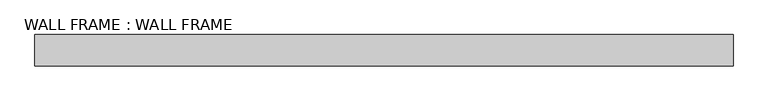
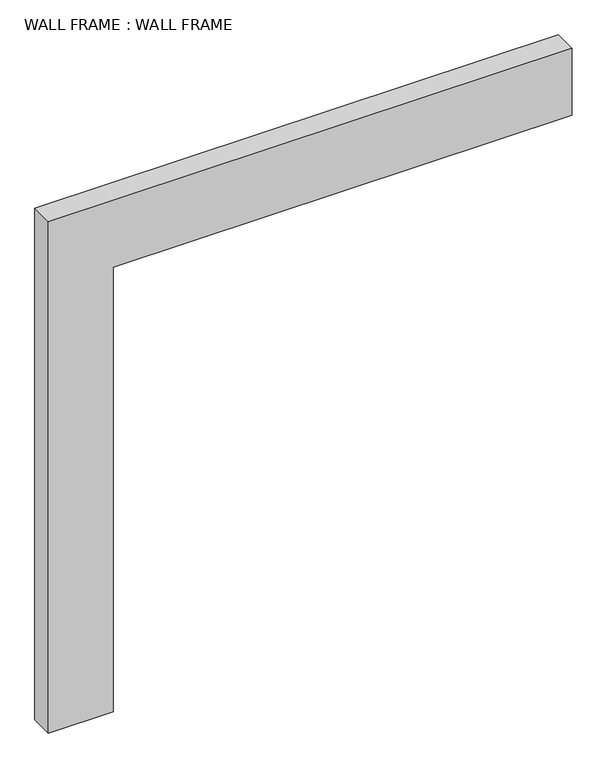
"""IFC4 building model written with IfcOpenShell, lengths in millimetres: proxy geometry, WALL FRAME : WALL FRAME."""

from ifc_helpers import new_model, si_unit, frame, origin, place, context, project, spatial, polyline, outline, extrude, source, transform, mapped, element, save


def wall_frame_wall_frame_a6ba02d1(model_context):
    return source(origin(), model_context, "Body", "SweptSolid", [
        extrude(outline(polyline([(7315.2, -7308.873248), (304.8, -7308.873248), (304.8, -6470.673248), (6400.8, -6470.673248), (6400.8, -514.373248), (7315.2, -514.373248), (7315.2, -7308.873248)])), frame((0.0, -4077.2866303, 0.0), z_axis=(0.0, 1.0, 0.0), x_axis=(0.0, 0.0, 1.0)), (0.0, 0.0, 1.0), 304.8),
    ])


if __name__ == "__main__":
    model = new_model("IFC4")
    model_context = context("Model", 3, world=origin())
    ifc_project = project(units=[si_unit("LENGTHUNIT", "METRE", prefix="MILLI")], contexts=[model_context])
    site = spatial("IfcSite", under=ifc_project)
    building = spatial("IfcBuilding", under=site)
    placement = place(None, origin())
    wall_frame_wall_frame_shape = wall_frame_wall_frame_a6ba02d1(model_context)
    element("IfcBuildingElementProxy", 1, Name="WALL FRAME : WALL FRAME", ObjectType="WALL FRAME : WALL FRAME", at=placement, inside=building, context=model_context, shape_type="MappedRepresentation", body=[
        mapped(wall_frame_wall_frame_shape, transform((0.0, 0.0, 0.0), x_axis=(1.0, 0.0, 0.0), y_axis=(0.0, 1.0, 0.0), z_axis=(0.0, 0.0, 1.0))),
    ])
    save(model, "model.ifc")

# Revit data of these elements
# Element 1 (IfcBuildingElementProxy, "WALL FRAME : WALL FRAME")
#   Materials on its faces: "WARM OFF WHITE"
# Materials
#   "WARM OFF WHITE": class "Generic", colour RGB 120 120 120, transparency 0, Cost = 0
